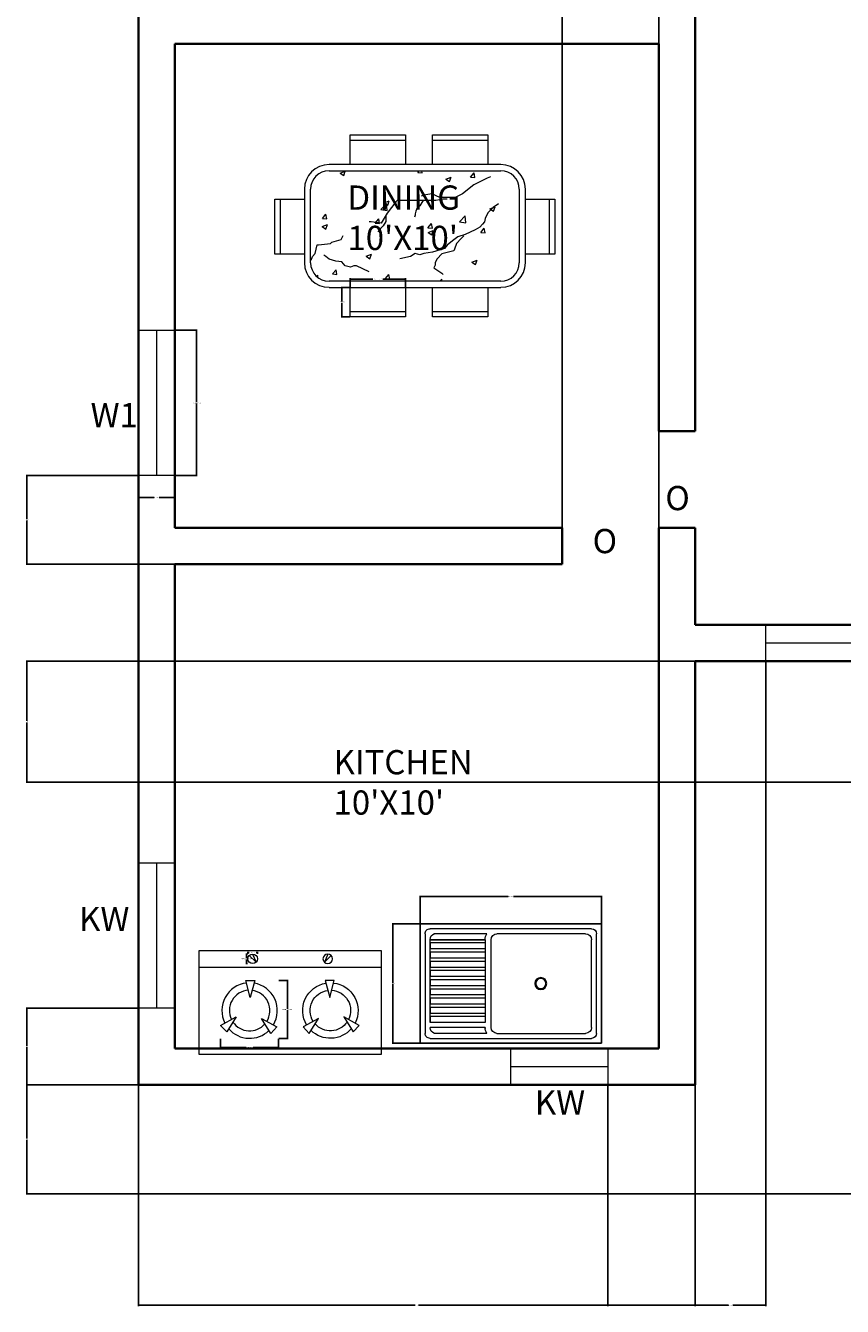
# Model space of a CAD drawing. Units: inches. Extents: x -4347 to -3836, y 955 to 1521.
# Tile 1 of 11: x -4347 to -4144, y 967 to 1284. Entities that reach past the tile are written whole.
import ezdxf

# ---------------------------------------------------------------- set-up
doc = ezdxf.new("R2010")
doc.units = ezdxf.units.IN
doc.header["$MEASUREMENT"] = 0
for name, color, linetype, lineweight in [('A-ANNO-DIMS', 2, 'Continuous', 18), ('A-ANNO-TEXT', 7, 'Continuous', 18), ('A-AREA-IDEN', 7, 'Continuous', 18), ('A-EQPM', 9, 'Continuous', 18), ('A-FLOR', 7, 'Continuous', 25), ('A-FLOR-FIXT', 9, 'Continuous', 18), ('A-FURN', 8, 'Continuous', 13), ('A-GLAZ', 4, 'Continuous', 18), ('A-WALL', 7, 'Continuous', 35)]:
    doc.layers.add(name, color=color, linetype=linetype, lineweight=lineweight)
doc.styles.get("Standard").update_dxf_attribs({"font": 'arial.ttf'})
doc.dimstyles.get("Standard").update_dxf_attribs({"dimtxt": 0.18, "dimasz": 0.18, "dimexe": 0.18, "dimexo": 0.0625, "dimgap": 0.09, "dimtad": 0, "dimtih": 1, "dimtoh": 1, "dimdec": 0, "dimzin": 0, "dimdsep": 46, "dimlunit": 3, "dimtxsty": 'Standard', "dimcen": 0.09, "dimadec": 0, "dimazin": 0, "dimtfac": 1, "dimtdec": 0, "dimtofl": 0, "dimtmove": 0, "dimatfit": 3, "dimfxl": 1, "dimtolj": 1, "dimtzin": 0, "dimarcsym": 0})

# ---------------------------------------------------------------- blocks, each defined once
blk = doc.blocks.new('М12 540х820')
for p, q in [((0, 540), (-820, 540)), ((-820, 540), (-820, 0)), ((0, 0), (0, 540)), ((-797.5, 495), (-797.5, 45)), ((-45, 517.5), (-775, 517.5)), ((-775, 468), (-775, 72)), ((-347.5, 495), (-748, 495)), ((-320.5, 468), (-320.5, 72)), ((-301.7, 495), (-64.8, 495)), ((-293.7, 468), (-293.7, 472.5)), ((-293.7, 468), (-45, 468)), ((-45, 469.5), (-45, 468)), ((-22.5, 45), (-22.5, 495)), ((-293.7, 446.6), (-45, 446.6)), ((-293.7, 419.6), (-293.7, 446.6)), ((-293.7, 419.6), (-45, 419.6)), ((-293.7, 405), (-45, 405)), ((-293.7, 378), (-293.7, 405)), ((-45, 419.6), (-45, 446.6)), ((-45, 378), (-45, 405)), ((-293.7, 378), (-45, 378)), ((-293.7, 336.4), (-293.7, 363.4)), ((-293.7, 363.4), (-45, 363.4)), ((-45, 336.4), (-45, 363.4)), ((-293.7, 336.4), (-45, 336.4)), ((-293.7, 294.7), (-293.7, 321.7)), ((-293.7, 321.7), (-45, 321.7)), ((-293.7, 294.7), (-45, 294.7)), ((-45, 294.7), (-45, 321.7)), ((-293.7, 253.1), (-293.7, 280.1)), ((-293.7, 280.1), (-45, 280.1)), ((-293.7, 253.1), (-45, 253.1)), ((-293.7, 211.5), (-293.7, 238.5)), ((-293.7, 238.5), (-45, 238.5)), ((-45, 253.1), (-45, 280.1)), ((-45, 211.5), (-45, 238.5)), ((-293.7, 211.5), (-45, 211.5)), ((-293.7, 169.9), (-293.7, 196.9)), ((-293.7, 196.9), (-45, 196.9)), ((-45, 169.9), (-45, 196.9)), ((-293.7, 169.9), (-45, 169.9)), ((-293.7, 128.2), (-293.7, 155.2)), ((-293.7, 155.2), (-45, 155.2)), ((-293.7, 128.2), (-45, 128.2)), ((-45, 128.2), (-45, 155.2)), ((-293.7, 113.6), (-45, 113.6)), ((-293.7, 86.6), (-293.7, 113.6)), ((-293.7, 86.6), (-45, 86.6)), ((-293.7, 72), (-45, 72)), ((-45, 86.6), (-45, 113.6)), ((-45, 70.5), (-45, 72)), ((-820, 0), (0, 0)), ((-775, 22.5), (-45, 22.5)), ((-748, 45), (-347.5, 45)), ((-301.7, 45), (-64.8, 45))]:
    blk.add_line(p, q)
at = {"ltscale": 0.06}
for p, q in [((-820, 0), (-820, 540)), ((-820, 540), (0, 540)), ((0, 540), (0, 536.9)), ((0, 536.9), (0, 0)), ((-293.7, 446.6), (-45, 446.6)), ((-293.7, 405), (-293.7, 446.6)), ((-293.7, 363.4), (-293.7, 405)), ((-45, 446.6), (-45, 419.6)), ((-45, 419.6), (-45, 378)), ((-293.7, 321.7), (-293.7, 363.4)), ((-45, 378), (-45, 336.4)), ((-293.7, 280.1), (-293.7, 321.7)), ((-45, 336.4), (-45, 294.7)), ((-45, 294.7), (-45, 253.1)), ((-293.7, 238.5), (-293.7, 280.1)), ((-293.7, 196.9), (-293.7, 238.5)), ((-45, 253.1), (-45, 211.5)), ((-293.7, 155.2), (-293.7, 196.9)), ((-45, 211.5), (-45, 169.9)), ((-293.7, 113.6), (-293.7, 155.2)), ((-45, 169.9), (-45, 128.2)), ((-45, 128.2), (-45, 86.6)), ((-293.7, 72), (-293.7, 113.6)), ((-45, 72), (-293.7, 72)), ((-45, 86.6), (-45, 72)), ((0, 0), (-820, 0))]:
    blk.add_line(p, q, dxfattribs=at)
at = {"extrusion": (0, 0, -1)}
for centre, major_axis, start_param, end_param in [((-775, 495), (-15.9, 15.9), -0.785398, 0.785398), ((-775, 495), (-15.9, 15.9), -0.785398, 0.785398), ((-748, 468), (-19.1, -19.1), 0.785398, 2.356194), ((-748, 468), (-19.1, -19.1), 0.785398, 2.356194), ((-347.5, 468), (-19.1, 19.1), 0.785398, 2.356194), ((-347.5, 468), (-19.1, 19.1), 0.785398, 2.356194), ((-343.2, 468), (-35, 35), 1.779263, 2.356194), ((-343.2, 468), (-35, 35), 1.779263, 2.356192), ((-343.2, 468), (-35, 35), 2.356192, 2.356194), ((-72.3, 468.8), (-19.3, 19.3), 1.0328, 2.38382), ((-72.3, 468.8), (-19.3, 19.3), 1.0328, 1.064673), ((-72.3, 468.8), (-19.3, 19.3), 1.064673, 2.328569), ((-45, 495), (-15.9, -15.9), 2.356194, 3.926991), ((-45, 495), (-15.9, -15.9), 2.356194, 3.926991), ((-72.3, 468.8), (-19.3, 19.3), 2.328569, 2.38382), ((-545.5, 270), (-19.1, -19.1), 3.926991, 10.210176), ((-545.5, 270), (-19.1, -19.1), 3.926991, 10.210176), ((-545.5, 270), (-15.9, -15.9), 3.926991, 10.210176), ((-545.5, 270), (-15.9, -15.9), 3.926991, 10.210176), ((-748, 72), (-19.1, 19.1), 3.926991, 5.497787), ((-748, 72), (-19.1, 19.1), 3.926991, 5.497787), ((-347.5, 72), (-19.1, -19.1), 3.926991, 5.497787), ((-347.5, 72), (-19.1, -19.1), 3.926991, 5.497787), ((-343.2, 72), (-35, -35), 3.926991, 4.503922), ((-343.2, 72), (-35, -35), 3.926991, 4.503922), ((-72.3, 71.2), (-19.3, -19.3), 3.899365, 5.250385), ((-72.3, 71.2), (-19.3, -19.3), 3.954617, 5.218512), ((-72.3, 71.2), (-19.3, -19.3), 3.899365, 3.954617), ((-775, 45), (-15.9, -15.9), 5.497787, 7.068583), ((-775, 45), (-15.9, -15.9), 5.497787, 7.068583), ((-72.3, 71.2), (-19.3, -19.3), 5.218512, 5.250385), ((-45, 45), (-15.9, 15.9), 2.356194, 3.926991), ((-45, 45), (-15.9, 15.9), 2.356194, 3.926991)]:
    blk.add_ellipse(centre, major_axis=major_axis, ratio=1, start_param=start_param, end_param=end_param, dxfattribs=at)
blk = doc.blocks.new('CHAIR-DINING')
for p, q in [((0, 0), (0, 7.33)), ((0, 7.33), (13.69, 7.33)), ((13.69, 7.33), (13.69, 0)), ((13.69, 5.99), (0, 5.99))]:
    blk.add_line(p, q)
blk = doc.blocks.new('GLAZ-24IN')
for p, q in [((0, 9), (24, 9)), ((0, 0), (0, 9)), ((24, 9), (24, 0)), ((0, 4.5), (24, 4.5)), ((24, 0), (0, 0))]:
    blk.add_line(p, q)
blk = doc.blocks.new('GLAZ-36IN')
for p, q in [((0, 0), (0, 36)), ((0, 36), (9, 36)), ((4.5, 36), (4.5, 0)), ((9, 36), (9, 0)), ((9, 0), (0, 0))]:
    blk.add_line(p, q)
blk = doc.blocks.new('GLAZ-60IN')
for p, q in [((0, 9), (60, 9)), ((0, 0), (0, 9)), ((60, 9), (60, 0)), ((0, 4.5), (60, 4.5)), ((60, 0), (0, 0))]:
    blk.add_line(p, q)
blk = doc.blocks.new('COOKTOP-BURNER')
for p, q in [((7.31, 10.12), (6.25, 14.36)), ((6.25, 14.36), (8.48, 14.36)), ((8.48, 14.36), (7.31, 10.12)), ((0, 3.2), (3.84, 5.33)), ((1.56, 1.61), (0, 3.2)), ((3.84, 5.33), (1.56, 1.61)), ((12.43, 1.2), (10.12, 4.94)), ((10.12, 4.94), (13.95, 2.83)), ((13.95, 2.83), (12.43, 1.2))]:
    blk.add_line(p, q)
for radius, start, end in [(6.87, 96.4005, 206.769), (6.87, 328.853, 80.7562), (5.03, 93.5753, 205.9207), (5.03, 327.9778, 83.02), (5.03, 214.5561, 318.8027), (6.87, 221.2225, 314.1627)]:
    blk.add_arc((7.18, 6.87), radius, start, end)
blk = doc.blocks.new('COOKTOP-CONTROL')
at = {"ltscale": 20}
for p, q in [((2.03, 0.35), (0.34, 2.02)), ((1.18, 2.37), (2.03, 0.35))]:
    blk.add_line(p, q, dxfattribs=at)
blk.add_circle((1.19, 1.19), 1.19, dxfattribs=at)
blk = doc.blocks.new('*D18')
at = {"layer": 'A-ANNO-DIMS', "color": 0, "lineweight": -2, "transparency": 16777216}
for p, q in [((-4266.08, 1219.49), (-4266.08, 1221.66)), ((-4265.9, 1221.48), (-4260.51, 1221.48)), ((-4252.57, 1221.48), (-4257.97, 1221.48)), ((-4252.39, 1219.49), (-4252.39, 1221.66))]:
    blk.add_line(p, q, dxfattribs=at)
at = {"layer": 'A-ANNO-DIMS', "color": 0, "transparency": 16777216}
for points in [[(-4265.9, 1221.51), (-4265.9, 1221.45), (-4266.08, 1221.48)], [(-4252.57, 1221.51), (-4252.57, 1221.45), (-4252.39, 1221.48)]]:
    blk.add_solid(points, dxfattribs=at)
at = {"layer": 'Defpoints', "color": 0, "transparency": 16777216}
for p in [(-4266.08, 1221.48), (-4266.08, 1219.42), (-4252.39, 1219.42)]:
    blk.add_point(p, dxfattribs=at)
at = {"layer": 'A-ANNO-DIMS', "color": 0, "transparency": 16777216, "insert": (-4259.24, 1221.48), "char_height": 0.18, "attachment_point": 5}
blk.add_mtext('\\A1;CHAIR 1\'-1 1/2" TYP.', dxfattribs=at)
blk = doc.blocks.new('*D19')
at = {"layer": 'A-ANNO-DIMS', "color": 0, "lineweight": -2, "transparency": 16777216}
for p, q in [((-4266.15, 1219.42), (-4268.32, 1219.42)), ((-4268.14, 1219.24), (-4268.14, 1215.94)), ((-4268.14, 1212.27), (-4268.14, 1215.57)), ((-4266.15, 1212.09), (-4268.32, 1212.09))]:
    blk.add_line(p, q, dxfattribs=at)
at = {"layer": 'A-ANNO-DIMS', "color": 0, "transparency": 16777216}
for points in [[(-4268.17, 1219.24), (-4268.11, 1219.24), (-4268.14, 1219.42)], [(-4268.17, 1212.27), (-4268.11, 1212.27), (-4268.14, 1212.09)]]:
    blk.add_solid(points, dxfattribs=at)
at = {"layer": 'Defpoints', "color": 0, "transparency": 16777216}
for p in [(-4266.08, 1219.42), (-4268.14, 1212.09), (-4266.08, 1212.09)]:
    blk.add_point(p, dxfattribs=at)
at = {"layer": 'A-ANNO-DIMS', "color": 0, "transparency": 16777216, "insert": (-4268.14, 1215.76), "char_height": 0.18, "attachment_point": 5}
blk.add_mtext('\\A1;0\'-7 1/2" TYP.', dxfattribs=at)
blk = doc.blocks.new('*D26')
at = {"layer": 'A-ANNO-DIMS', "color": 0, "lineweight": -2, "transparency": 16777216}
for p, q in [((-4309.52, 1208.78), (-4304, 1208.78)), ((-4304.18, 1208.6), (-4304.18, 1190.97)), ((-4304.18, 1172.96), (-4304.18, 1190.6)), ((-4309.52, 1172.78), (-4304, 1172.78))]:
    blk.add_line(p, q, dxfattribs=at)
at = {"layer": 'A-ANNO-DIMS', "color": 0, "transparency": 16777216}
for points in [[(-4304.21, 1208.6), (-4304.15, 1208.6), (-4304.18, 1208.78)], [(-4304.21, 1172.96), (-4304.15, 1172.96), (-4304.18, 1172.78)]]:
    blk.add_solid(points, dxfattribs=at)
at = {"layer": 'Defpoints', "color": 0, "transparency": 16777216}
for p in [(-4309.58, 1208.78), (-4304.18, 1208.78), (-4309.58, 1172.78)]:
    blk.add_point(p, dxfattribs=at)
at = {"layer": 'A-ANNO-DIMS', "color": 0, "transparency": 16777216, "insert": (-4304.18, 1190.78), "char_height": 0.18, "attachment_point": 5}
blk.add_mtext('\\A1;GLAZING 3\'-0" TYP.', dxfattribs=at)
blk = doc.blocks.new('*D27')
at = {"layer": 'A-ANNO-DIMS', "color": 0, "lineweight": -2, "transparency": 16777216}
for p, q in [((-4318.58, 1172.72), (-4318.58, 1167.2)), ((-4309.58, 1172.72), (-4309.58, 1167.2)), ((-4318.4, 1167.38), (-4314.72, 1167.38)), ((-4309.76, 1167.38), (-4313.44, 1167.38))]:
    blk.add_line(p, q, dxfattribs=at)
at = {"layer": 'A-ANNO-DIMS', "color": 0, "transparency": 16777216}
for points in [[(-4318.4, 1167.41), (-4318.4, 1167.35), (-4318.58, 1167.38)], [(-4309.76, 1167.41), (-4309.76, 1167.35), (-4309.58, 1167.38)]]:
    blk.add_solid(points, dxfattribs=at)
at = {"layer": 'Defpoints', "color": 0, "transparency": 16777216}
for p in [(-4318.58, 1172.78), (-4309.58, 1172.78), (-4309.58, 1167.38)]:
    blk.add_point(p, dxfattribs=at)
at = {"layer": 'A-ANNO-DIMS', "color": 0, "transparency": 16777216, "insert": (-4314.08, 1167.38), "char_height": 0.18, "attachment_point": 5}
blk.add_mtext('\\A1;0\'-9" TYP.', dxfattribs=at)
blk = doc.blocks.new('*D30')
at = {"layer": 'A-ANNO-DIMS', "color": 0, "lineweight": -2, "transparency": 16777216}
for p, q in [((-4283.77, 1047.67), (-4281.48, 1047.67)), ((-4281.66, 1047.49), (-4281.66, 1040.63)), ((-4281.66, 1033.41), (-4281.66, 1040.27)), ((-4283.77, 1033.23), (-4281.48, 1033.23))]:
    blk.add_line(p, q, dxfattribs=at)
at = {"layer": 'A-ANNO-DIMS', "color": 0, "transparency": 16777216}
for points in [[(-4281.69, 1047.49), (-4281.63, 1047.49), (-4281.66, 1047.67)], [(-4281.69, 1033.41), (-4281.63, 1033.41), (-4281.66, 1033.23)]]:
    blk.add_solid(points, dxfattribs=at)
at = {"layer": 'Defpoints', "color": 0, "transparency": 16777216}
for p in [(-4283.83, 1047.67), (-4281.66, 1047.67), (-4283.83, 1033.23)]:
    blk.add_point(p, dxfattribs=at)
at = {"layer": 'A-ANNO-DIMS', "color": 0, "transparency": 16777216, "insert": (-4281.66, 1040.45), "char_height": 0.18, "attachment_point": 5}
blk.add_mtext('\\A1;BURNER 1\'-2 1/2" TYP.', dxfattribs=at)
blk = doc.blocks.new('*D31')
at = {"layer": 'A-ANNO-DIMS', "color": 0, "lineweight": -2, "transparency": 16777216}
for p, q in [((-4298.21, 1033.17), (-4298.21, 1030.89)), ((-4283.83, 1033.17), (-4283.83, 1030.89)), ((-4298.03, 1031.07), (-4291.86, 1031.07)), ((-4284.01, 1031.07), (-4290.18, 1031.07))]:
    blk.add_line(p, q, dxfattribs=at)
at = {"layer": 'A-ANNO-DIMS', "color": 0, "transparency": 16777216}
for points in [[(-4298.03, 1031.1), (-4298.03, 1031.04), (-4298.21, 1031.07)], [(-4284.01, 1031.1), (-4284.01, 1031.04), (-4283.83, 1031.07)]]:
    blk.add_solid(points, dxfattribs=at)
at = {"layer": 'Defpoints', "color": 0, "transparency": 16777216}
for p in [(-4298.21, 1033.23), (-4283.83, 1033.23), (-4283.83, 1031.07)]:
    blk.add_point(p, dxfattribs=at)
at = {"layer": 'A-ANNO-DIMS', "color": 0, "transparency": 16777216, "insert": (-4291.02, 1031.07), "char_height": 0.18, "attachment_point": 5}
blk.add_mtext('\\A1;1\'-2 1/2" TYP.', dxfattribs=at)
blk = doc.blocks.new('*D32')
at = {"layer": 'A-ANNO-DIMS', "color": 0, "lineweight": -2, "transparency": 16777216}
for p, q in [((-4291.53, 1054.2), (-4292.01, 1054.2)), ((-4291.83, 1054.02), (-4291.83, 1053.19)), ((-4291.53, 1051.82), (-4292.01, 1051.82)), ((-4291.83, 1052), (-4291.83, 1052.83))]:
    blk.add_line(p, q, dxfattribs=at)
at = {"layer": 'A-ANNO-DIMS', "color": 0, "transparency": 16777216}
for points in [[(-4291.86, 1054.02), (-4291.8, 1054.02), (-4291.83, 1054.2)], [(-4291.86, 1052), (-4291.8, 1052), (-4291.83, 1051.82)]]:
    blk.add_solid(points, dxfattribs=at)
at = {"layer": 'Defpoints', "color": 0, "transparency": 16777216}
for p in [(-4291.83, 1054.2), (-4291.47, 1054.2), (-4291.47, 1051.82)]:
    blk.add_point(p, dxfattribs=at)
at = {"layer": 'A-ANNO-DIMS', "color": 0, "transparency": 16777216, "insert": (-4291.83, 1053.01), "char_height": 0.18, "attachment_point": 5}
blk.add_mtext('\\A1;CONTROL 0\'-2 1/2" TYP.', dxfattribs=at)
blk = doc.blocks.new('*D33')
at = {"layer": 'A-ANNO-DIMS', "color": 0, "lineweight": -2, "transparency": 16777216}
for p, q in [((-4291.47, 1054.26), (-4291.47, 1054.73)), ((-4291.29, 1054.55), (-4291.13, 1054.55)), ((-4289.28, 1054.55), (-4289.44, 1054.55)), ((-4289.1, 1054.26), (-4289.1, 1054.73))]:
    blk.add_line(p, q, dxfattribs=at)
at = {"layer": 'A-ANNO-DIMS', "color": 0, "transparency": 16777216}
for points in [[(-4291.29, 1054.58), (-4291.29, 1054.52), (-4291.47, 1054.55)], [(-4289.28, 1054.58), (-4289.28, 1054.52), (-4289.1, 1054.55)]]:
    blk.add_solid(points, dxfattribs=at)
at = {"layer": 'Defpoints', "color": 0, "transparency": 16777216}
for p in [(-4291.47, 1054.2), (-4289.1, 1054.55), (-4289.1, 1054.2)]:
    blk.add_point(p, dxfattribs=at)
at = {"layer": 'A-ANNO-DIMS', "color": 0, "transparency": 16777216, "insert": (-4290.28, 1054.55), "char_height": 0.18, "attachment_point": 5}
blk.add_mtext('\\A1;0\'-2 1/2" TYP.', dxfattribs=at)
blk = doc.blocks.new('*D34')
at = {"layer": 'A-ANNO-DIMS', "color": 0, "lineweight": -2, "transparency": 16777216}
for p, q in [((-4248.77, 1061.76), (-4248.77, 1068.63)), ((-4248.59, 1068.45), (-4226.92, 1068.45)), ((-4203.95, 1068.45), (-4225.61, 1068.45)), ((-4203.77, 1061.76), (-4203.77, 1068.63))]:
    blk.add_line(p, q, dxfattribs=at)
at = {"layer": 'A-ANNO-DIMS', "color": 0, "transparency": 16777216}
for points in [[(-4248.59, 1068.48), (-4248.59, 1068.42), (-4248.77, 1068.45)], [(-4203.95, 1068.48), (-4203.95, 1068.42), (-4203.77, 1068.45)]]:
    blk.add_solid(points, dxfattribs=at)
at = {"layer": 'Defpoints', "color": 0, "transparency": 16777216}
for p in [(-4248.77, 1068.45), (-4248.77, 1061.7), (-4203.77, 1061.7)]:
    blk.add_point(p, dxfattribs=at)
at = {"layer": 'A-ANNO-DIMS', "color": 0, "transparency": 16777216, "insert": (-4226.27, 1068.45), "char_height": 0.18, "attachment_point": 5}
blk.add_mtext('\\A1;SINK 3\'-9"', dxfattribs=at)
blk = doc.blocks.new('*D35')
at = {"layer": 'A-ANNO-DIMS', "color": 0, "lineweight": -2, "transparency": 16777216}
for p, q in [((-4248.83, 1061.7), (-4255.7, 1061.7)), ((-4255.52, 1061.52), (-4255.52, 1047.07)), ((-4255.52, 1032.25), (-4255.52, 1046.7)), ((-4248.83, 1032.07), (-4255.7, 1032.07))]:
    blk.add_line(p, q, dxfattribs=at)
at = {"layer": 'A-ANNO-DIMS', "color": 0, "transparency": 16777216}
for points in [[(-4255.55, 1061.52), (-4255.49, 1061.52), (-4255.52, 1061.7)], [(-4255.55, 1032.25), (-4255.49, 1032.25), (-4255.52, 1032.07)]]:
    blk.add_solid(points, dxfattribs=at)
at = {"layer": 'Defpoints', "color": 0, "transparency": 16777216}
for p in [(-4248.77, 1061.7), (-4255.52, 1032.07), (-4248.77, 1032.07)]:
    blk.add_point(p, dxfattribs=at)
at = {"layer": 'A-ANNO-DIMS', "color": 0, "transparency": 16777216, "insert": (-4255.52, 1046.88), "char_height": 0.18, "attachment_point": 5}
blk.add_mtext('\\A1;2\'-5 1/2"', dxfattribs=at)
blk = doc.blocks.new('*D39')
at = {"layer": 'A-ANNO-DIMS', "color": 0, "lineweight": -2, "transparency": 16777216}
for p, q in [((-4318.58, 1021.73), (-4318.58, 966.96)), ((-4180.58, 1021.73), (-4180.58, 966.96)), ((-4318.4, 967.14), (-4249.97, 967.14)), ((-4180.76, 967.14), (-4249.19, 967.14))]:
    blk.add_line(p, q, dxfattribs=at)
at = {"layer": 'A-ANNO-DIMS', "color": 0, "transparency": 16777216}
for points in [[(-4318.4, 967.17), (-4318.4, 967.11), (-4318.58, 967.14)], [(-4180.76, 967.17), (-4180.76, 967.11), (-4180.58, 967.14)]]:
    blk.add_solid(points, dxfattribs=at)
at = {"layer": 'Defpoints', "color": 0, "transparency": 16777216}
for p in [(-4318.58, 1021.79), (-4180.58, 1021.79), (-4180.58, 967.14)]:
    blk.add_point(p, dxfattribs=at)
at = {"layer": 'A-ANNO-DIMS', "color": 0, "transparency": 16777216, "insert": (-4249.58, 967.14), "char_height": 0.18, "attachment_point": 5}
blk.add_mtext('\\A1;11\'-6"', dxfattribs=at)
blk = doc.blocks.new('*D40')
at = {"layer": 'A-ANNO-DIMS', "color": 0, "lineweight": -2, "transparency": 16777216}
for p, q in [((-4318.64, 1021.79), (-4346.41, 1021.79)), ((-4346.23, 1021.61), (-4346.23, 1008.47)), ((-4346.23, 994.97), (-4346.23, 1008.11)), ((-4180.64, 994.79), (-4346.41, 994.79))]:
    blk.add_line(p, q, dxfattribs=at)
at = {"layer": 'A-ANNO-DIMS', "color": 0, "transparency": 16777216}
for points in [[(-4346.26, 1021.61), (-4346.2, 1021.61), (-4346.23, 1021.79)], [(-4346.26, 994.97), (-4346.2, 994.97), (-4346.23, 994.79)]]:
    blk.add_solid(points, dxfattribs=at)
at = {"layer": 'Defpoints', "color": 0, "transparency": 16777216}
for p in [(-4346.23, 1021.79), (-4318.58, 1021.79), (-4180.58, 994.79)]:
    blk.add_point(p, dxfattribs=at)
at = {"layer": 'A-ANNO-DIMS', "color": 0, "transparency": 16777216, "insert": (-4346.23, 1008.29), "char_height": 0.18, "attachment_point": 5}
blk.add_mtext('\\A1;2\'-3"', dxfattribs=at)
blk = doc.blocks.new('*D41')
at = {"layer": 'A-ANNO-DIMS', "color": 0, "lineweight": -2, "transparency": 16777216}
for p, q in [((-4318.64, 1040.78), (-4346.41, 1040.78)), ((-4346.23, 1040.6), (-4346.23, 1031.46)), ((-4346.23, 1021.97), (-4346.23, 1031.1)), ((-4318.64, 1021.79), (-4346.41, 1021.79))]:
    blk.add_line(p, q, dxfattribs=at)
at = {"layer": 'A-ANNO-DIMS', "color": 0, "transparency": 16777216}
for points in [[(-4346.26, 1040.6), (-4346.2, 1040.6), (-4346.23, 1040.78)], [(-4346.26, 1021.97), (-4346.2, 1021.97), (-4346.23, 1021.79)]]:
    blk.add_solid(points, dxfattribs=at)
at = {"layer": 'Defpoints', "color": 0, "transparency": 16777216}
for p in [(-4346.23, 1040.78), (-4318.58, 1040.78), (-4318.58, 1021.79)]:
    blk.add_point(p, dxfattribs=at)
at = {"layer": 'A-ANNO-DIMS', "color": 0, "transparency": 16777216, "insert": (-4346.23, 1031.28), "char_height": 0.18, "attachment_point": 5}
blk.add_mtext('\\A1;1\'-7"', dxfattribs=at)
blk = doc.blocks.new('*D42')
at = {"layer": 'A-ANNO-DIMS', "color": 0, "lineweight": -2, "transparency": 16777216}
for p, q in [((-4318.64, 1172.78), (-4346.41, 1172.78)), ((-4346.23, 1172.6), (-4346.23, 1161.97)), ((-4346.23, 1150.97), (-4346.23, 1161.6)), ((-4309.64, 1150.79), (-4346.41, 1150.79))]:
    blk.add_line(p, q, dxfattribs=at)
at = {"layer": 'A-ANNO-DIMS', "color": 0, "transparency": 16777216}
for points in [[(-4346.26, 1172.6), (-4346.2, 1172.6), (-4346.23, 1172.78)], [(-4346.26, 1150.97), (-4346.2, 1150.97), (-4346.23, 1150.79)]]:
    blk.add_solid(points, dxfattribs=at)
at = {"layer": 'Defpoints', "color": 0, "transparency": 16777216}
for p in [(-4346.23, 1172.78), (-4318.58, 1172.78), (-4309.58, 1150.79)]:
    blk.add_point(p, dxfattribs=at)
at = {"layer": 'A-ANNO-DIMS', "color": 0, "transparency": 16777216, "insert": (-4346.23, 1161.79), "char_height": 0.18, "attachment_point": 5}
blk.add_mtext('\\A1;1\'-10"', dxfattribs=at)
blk = doc.blocks.new('*D46')
at = {"layer": 'A-ANNO-DIMS', "color": 0, "lineweight": -2, "transparency": 16777216}
for p, q in [((-4202.26, 1021.73), (-4202.26, 966.96)), ((-4180.58, 1021.73), (-4180.58, 966.96)), ((-4202.08, 967.14), (-4191.95, 967.14)), ((-4180.76, 967.14), (-4190.89, 967.14))]:
    blk.add_line(p, q, dxfattribs=at)
at = {"layer": 'A-ANNO-DIMS', "color": 0, "transparency": 16777216}
for points in [[(-4202.08, 967.17), (-4202.08, 967.11), (-4202.26, 967.14)], [(-4180.76, 967.17), (-4180.76, 967.11), (-4180.58, 967.14)]]:
    blk.add_solid(points, dxfattribs=at)
at = {"layer": 'Defpoints', "color": 0, "transparency": 16777216}
for p in [(-4202.26, 1021.79), (-4180.58, 1021.79), (-4180.58, 967.14)]:
    blk.add_point(p, dxfattribs=at)
at = {"layer": 'A-ANNO-DIMS', "color": 0, "transparency": 16777216, "insert": (-4191.42, 967.14), "char_height": 0.18, "attachment_point": 5}
blk.add_mtext('\\A1;1\'-9 1/2"', dxfattribs=at)
blk = doc.blocks.new('*D54')
at = {"layer": 'A-ANNO-DIMS', "color": 0, "lineweight": -2, "transparency": 16777216}
for p, q in [((-3997.76, 1126.79), (-4346.41, 1126.79)), ((-4346.23, 1126.61), (-4346.23, 1111.97)), ((-4346.23, 1096.97), (-4346.23, 1111.61)), ((-3997.76, 1096.79), (-4346.41, 1096.79))]:
    blk.add_line(p, q, dxfattribs=at)
at = {"layer": 'A-ANNO-DIMS', "color": 0, "transparency": 16777216}
for points in [[(-4346.26, 1126.61), (-4346.2, 1126.61), (-4346.23, 1126.79)], [(-4346.26, 1096.97), (-4346.2, 1096.97), (-4346.23, 1096.79)]]:
    blk.add_solid(points, dxfattribs=at)
at = {"layer": 'Defpoints', "color": 0, "transparency": 16777216}
for p in [(-4346.23, 1126.79), (-3997.69, 1126.79), (-3997.69, 1096.79)]:
    blk.add_point(p, dxfattribs=at)
at = {"layer": 'A-ANNO-DIMS', "color": 0, "transparency": 16777216, "insert": (-4346.23, 1111.79), "char_height": 0.18, "attachment_point": 5}
blk.add_mtext('\\A1;2\'-6"', dxfattribs=at)
blk = doc.blocks.new('*D56')
at = {"layer": 'A-ANNO-DIMS', "color": 0, "lineweight": -2, "transparency": 16777216}
for p, q in [((-4180.58, 1126.73), (-4180.58, 966.96)), ((-4163.03, 1126.73), (-4163.03, 966.96)), ((-4180.4, 967.14), (-4172.34, 967.14)), ((-4163.21, 967.14), (-4171.27, 967.14))]:
    blk.add_line(p, q, dxfattribs=at)
at = {"layer": 'A-ANNO-DIMS', "color": 0, "transparency": 16777216}
for points in [[(-4180.4, 967.17), (-4180.4, 967.11), (-4180.58, 967.14)], [(-4163.21, 967.17), (-4163.21, 967.11), (-4163.03, 967.14)]]:
    blk.add_solid(points, dxfattribs=at)
at = {"layer": 'Defpoints', "color": 0, "transparency": 16777216}
for p in [(-4180.58, 1126.79), (-4163.03, 1126.79), (-4163.03, 967.14)]:
    blk.add_point(p, dxfattribs=at)
at = {"layer": 'A-ANNO-DIMS', "color": 0, "transparency": 16777216, "insert": (-4171.81, 967.14), "char_height": 0.18, "attachment_point": 5}
blk.add_mtext('\\A1;1\'-5 1/2"', dxfattribs=at)
blk = doc.blocks.new('*D58')
at = {"layer": 'A-ANNO-DIMS', "color": 0, "lineweight": -2, "transparency": 16777216}
for p, q in [((-4213.58, 1159.85), (-4213.58, 1517.62)), ((-4213.4, 1517.44), (-4201.91, 1517.44)), ((-4189.76, 1517.44), (-4201.25, 1517.44)), ((-4189.58, 1159.85), (-4189.58, 1517.62))]:
    blk.add_line(p, q, dxfattribs=at)
at = {"layer": 'A-ANNO-DIMS', "color": 0, "transparency": 16777216}
for points in [[(-4213.4, 1517.47), (-4213.4, 1517.41), (-4213.58, 1517.44)], [(-4189.76, 1517.47), (-4189.76, 1517.41), (-4189.58, 1517.44)]]:
    blk.add_solid(points, dxfattribs=at)
at = {"layer": 'Defpoints', "color": 0, "transparency": 16777216}
for p in [(-4189.58, 1517.44), (-4213.58, 1159.79), (-4189.58, 1159.79)]:
    blk.add_point(p, dxfattribs=at)
at = {"layer": 'A-ANNO-DIMS', "color": 0, "transparency": 16777216, "insert": (-4201.58, 1517.44), "char_height": 0.18, "attachment_point": 5}
blk.add_mtext('\\A1;2\'-0"', dxfattribs=at)

msp = doc.modelspace()

# ---------------------------------------------------------------- linework, layer by layer
at = {"layer": 'A-EQPM'}
msp.add_line((-4303.51, 1050.91), (-4258.42, 1050.91), dxfattribs=at)
msp.add_lwpolyline([(-4258.42, 1029.33), (-4303.51, 1029.33), (-4303.51, 1055.1), (-4258.42, 1055.1)], close=True, dxfattribs=at)
at = {"layer": 'A-FLOR'}
for p, q in [((-4180.58, 1021.79), (-4180.58, 994.79)), ((-4180.58, 994.79), (-3931.58, 994.79))]:
    msp.add_line(p, q, dxfattribs=at)
at = {"layer": 'A-FURN'}
for p, q in [((-4228.75, 1249.85), (-4271.35, 1249.85)), ((-4271.35, 1248.33), (-4228.75, 1248.33)), ((-4268.58, 1247.72), (-4267.31, 1248.21)), ((-4268.58, 1247.72), (-4267.68, 1247.11)), ((-4267.68, 1247.11), (-4267.31, 1248.21)), ((-4249.34, 1247.91), (-4248.99, 1248.33)), ((-4249.34, 1247.91), (-4248.25, 1247.81)), ((-4248.25, 1247.81), (-4248.35, 1248.33)), ((-4236.25, 1246.76), (-4235.37, 1247.81)), ((-4235.16, 1246.67), (-4235.37, 1247.81)), ((-4242.35, 1246.26), (-4241.07, 1246.75)), ((-4242.35, 1246.26), (-4241.44, 1245.64)), ((-4241.44, 1245.64), (-4241.07, 1246.75)), ((-4235.44, 1244.87), (-4238.25, 1242.56)), ((-4236.25, 1246.76), (-4235.16, 1246.67)), ((-4232.13, 1246.52), (-4235.44, 1244.87)), ((-4231.3, 1246.85), (-4232.13, 1246.52)), ((-4277.43, 1243.76), (-4277.43, 1225.51)), ((-4275.91, 1225.51), (-4275.91, 1243.76)), ((-4247.84, 1242.23), (-4248.5, 1242.06)), ((-4245.86, 1242.56), (-4247.84, 1242.23)), ((-4243.87, 1241.73), (-4245.86, 1242.56)), ((-4243.05, 1241.24), (-4244.86, 1240.91)), ((-4240.07, 1241.73), (-4243.87, 1241.73)), ((-4242.05, 1241.24), (-4243.05, 1241.24)), ((-4238.25, 1242.56), (-4240.07, 1241.73)), ((-4224.19, 1243.76), (-4224.19, 1225.51)), ((-4222.67, 1225.51), (-4222.67, 1243.76)), ((-4258.51, 1238.71), (-4257.09, 1240.19)), ((-4258.51, 1238.71), (-4256.89, 1238.46)), ((-4257.69, 1240.37), (-4256.41, 1240.86)), ((-4257.69, 1240.37), (-4256.78, 1239.76)), ((-4256.89, 1238.46), (-4257.09, 1240.19)), ((-4254.79, 1240.58), (-4256.94, 1237.77)), ((-4256.78, 1239.76), (-4256.41, 1240.86)), ((-4254.46, 1240.91), (-4254.79, 1240.58)), ((-4244.86, 1240.91), (-4254.46, 1240.91)), ((-4249.83, 1238.27), (-4249.99, 1237.61)), ((-4249.49, 1239.09), (-4249.83, 1238.27)), ((-4248.83, 1239.59), (-4249.49, 1239.09)), ((-4248.34, 1240.42), (-4248.83, 1239.59)), ((-4248.01, 1240.91), (-4248.34, 1240.42)), ((-4231.96, 1237.93), (-4232.62, 1236.45)), ((-4230.64, 1239.25), (-4231.96, 1237.93)), ((-4231.45, 1238.91), (-4230.18, 1239.4)), ((-4231.45, 1238.91), (-4230.55, 1238.29)), ((-4229.32, 1240.08), (-4230.64, 1239.25)), ((-4230.55, 1238.29), (-4230.18, 1239.4)), ((-4273.03, 1234.48), (-4271.75, 1234.97)), ((-4273, 1236.47), (-4272.12, 1237.52)), ((-4273, 1236.47), (-4271.91, 1236.37)), ((-4271.91, 1236.37), (-4272.12, 1237.52)), ((-4272.12, 1233.87), (-4271.75, 1234.97)), ((-4260.91, 1235.62), (-4261.41, 1235.62)), ((-4258.43, 1235.29), (-4260.91, 1235.62)), ((-4259.9, 1235.32), (-4259.02, 1236.37)), ((-4259.9, 1235.32), (-4258.81, 1235.23)), ((-4258.81, 1235.23), (-4259.02, 1236.37)), ((-4256.94, 1237.77), (-4258.43, 1235.29)), ((-4257.27, 1235.78), (-4257.93, 1234.63)), ((-4257.27, 1237.27), (-4257.27, 1235.78)), ((-4249.99, 1237.28), (-4250.16, 1236.78)), ((-4249.99, 1237.61), (-4249.99, 1237.28)), ((-4246.81, 1234.18), (-4245.93, 1235.23)), ((-4245.72, 1234.08), (-4245.93, 1235.22)), ((-4239.03, 1235.69), (-4237.6, 1237.17)), ((-4239.03, 1235.69), (-4237.4, 1235.44)), ((-4237.4, 1235.44), (-4237.6, 1237.17)), ((-4233.29, 1235.12), (-4233.95, 1234.3)), ((-4232.79, 1235.62), (-4233.29, 1235.12)), ((-4232.62, 1236.45), (-4232.79, 1235.62)), ((-4273.03, 1234.48), (-4272.12, 1233.87)), ((-4268.35, 1231.32), (-4267.86, 1232.31)), ((-4258.59, 1233.97), (-4259.26, 1233.14)), ((-4257.93, 1234.63), (-4258.59, 1233.97)), ((-4246.81, 1234.18), (-4245.72, 1234.08)), ((-4246.79, 1233.02), (-4245.51, 1233.51)), ((-4246.79, 1233.02), (-4245.88, 1232.41)), ((-4245.88, 1232.41), (-4245.51, 1233.51)), ((-4239.41, 1231.98), (-4240.73, 1230.99)), ((-4237.59, 1232.48), (-4239.41, 1231.98)), ((-4237.92, 1232.15), (-4238.58, 1231.49)), ((-4235.11, 1233.64), (-4237.59, 1232.48)), ((-4233.95, 1234.3), (-4235.11, 1233.64)), ((-4233.72, 1233.03), (-4232.84, 1234.08)), ((-4233.72, 1233.03), (-4232.63, 1232.94)), ((-4232.62, 1232.93), (-4232.84, 1234.08)), ((-4274.8, 1227.85), (-4274.31, 1230)), ((-4274.31, 1230), (-4273.98, 1230)), ((-4273.98, 1230), (-4271, 1230.33)), ((-4271, 1230.33), (-4270.67, 1230.66)), ((-4270.67, 1230.66), (-4268.35, 1231.32)), ((-4242.71, 1229.01), (-4245.69, 1228.18)), ((-4240.4, 1228.51), (-4243.38, 1227.69)), ((-4242.05, 1229.84), (-4242.71, 1229.01)), ((-4240.73, 1230.99), (-4242.05, 1229.84)), ((-4240.23, 1228.85), (-4240.4, 1228.51)), ((-4239.74, 1230.33), (-4240.23, 1228.85)), ((-4238.58, 1231.49), (-4239.74, 1230.33)), ((-4275.8, 1226.2), (-4275.47, 1227.03)), ((-4275.47, 1227.03), (-4274.8, 1227.85)), ((-4272.16, 1227.03), (-4272.65, 1227.36)), ((-4271.33, 1226.37), (-4272.16, 1227.03)), ((-4269.67, 1225.88), (-4271.33, 1226.37)), ((-4268.19, 1225.71), (-4269.67, 1225.88)), ((-4267.36, 1224.72), (-4268.19, 1225.71)), ((-4262.13, 1227.13), (-4260.85, 1227.62)), ((-4262.13, 1227.13), (-4261.22, 1226.52)), ((-4261.22, 1226.52), (-4260.85, 1227.62)), ((-4251.15, 1227.03), (-4253.8, 1226.53)), ((-4249.99, 1227.85), (-4251.15, 1227.03)), ((-4248.83, 1227.52), (-4249.99, 1227.85)), ((-4247.84, 1227.85), (-4248.83, 1227.52)), ((-4245.69, 1228.18), (-4247.84, 1227.85)), ((-4244.53, 1226.53), (-4245.03, 1225.54)), ((-4245.03, 1225.54), (-4245.03, 1224.88)), ((-4243.38, 1227.69), (-4244.53, 1226.53)), ((-4235.9, 1225.67), (-4234.62, 1226.16)), ((-4235.9, 1225.67), (-4234.99, 1225.06)), ((-4234.99, 1225.06), (-4234.62, 1226.16)), ((-4274.42, 1222.13), (-4274.15, 1222.41)), ((-4274.08, 1221.86), (-4274.15, 1222.41)), ((-4270.46, 1222.74), (-4269.58, 1223.79)), ((-4270.46, 1222.74), (-4269.37, 1222.64)), ((-4269.37, 1222.64), (-4269.58, 1223.78)), ((-4266.04, 1224.39), (-4267.36, 1224.72)), ((-4265.21, 1224.72), (-4266.04, 1224.39)), ((-4264.55, 1224.72), (-4265.21, 1224.72)), ((-4261.4, 1223.23), (-4264.55, 1224.72)), ((-4257.37, 1221.59), (-4256.49, 1222.64)), ((-4256.28, 1221.49), (-4256.49, 1222.64)), ((-4245.03, 1224.88), (-4245.36, 1224.22)), ((-4245.36, 1224.22), (-4243.38, 1222.9)), ((-4243.38, 1222.9), (-4243.05, 1222.57)), ((-4228.75, 1220.94), (-4271.35, 1220.94)), ((-4271.35, 1219.42), (-4228.75, 1219.42)), ((-4257.37, 1221.59), (-4256.28, 1221.5)), ((-4243.86, 1220.94), (-4243.4, 1221.49)), ((-4243.3, 1220.94), (-4243.4, 1221.49))]:
    msp.add_line(p, q, dxfattribs=at)
for centre, radius, start, end in [((-4271.35, 1243.76), 6.08, 90, 180), ((-4271.35, 1243.76), 4.56, 90, 180), ((-4228.75, 1243.76), 6.08, 0, 90), ((-4228.75, 1243.76), 4.56, 0, 90), ((-4271.35, 1225.51), 6.08, 180, 270), ((-4271.35, 1225.51), 4.56, 180, 270), ((-4228.75, 1225.51), 4.56, 270, 0), ((-4228.75, 1225.51), 6.08, 270, 0)]:
    msp.add_arc(centre, radius, start, end, dxfattribs=at)
at = {"layer": 'A-WALL'}
for p, q in [((-4318.58, 1489.79), (-4318.58, 1021.79)), ((-4180.58, 1348.79), (-4180.58, 1183.79)), ((-4309.58, 1279.79), (-4189.58, 1279.79)), ((-4309.58, 1279.79), (-4309.58, 1159.79)), ((-4189.58, 1279.79), (-4189.58, 1183.79)), ((-4180.58, 1183.79), (-4189.58, 1183.79)), ((-4309.58, 1159.79), (-4213.58, 1159.79)), ((-4213.58, 1159.79), (-4213.58, 1150.79)), ((-4189.58, 1159.79), (-4180.58, 1159.79)), ((-4189.58, 1159.79), (-4189.58, 1030.79)), ((-4180.58, 1159.79), (-4180.58, 1135.79)), ((-4309.58, 1150.79), (-4213.58, 1150.79)), ((-4309.58, 1150.79), (-4309.58, 1030.79)), ((-4180.58, 1135.79), (-3976.58, 1135.79)), ((-4180.58, 1126.79), (-3976.58, 1126.79)), ((-4180.58, 1126.79), (-4180.58, 1021.79)), ((-4309.58, 1030.79), (-4189.58, 1030.79)), ((-4318.58, 1021.79), (-4180.58, 1021.79))]:
    msp.add_line(p, q, dxfattribs=at)

# ---------------------------------------------------------------- block references
at = {"layer": 'A-EQPM'}
for name, p in [('COOKTOP-CONTROL', (-4291.47, 1051.82)), ('COOKTOP-BURNER', (-4298.21, 1033.31))]:
    msp.add_blockref(name, p, dxfattribs=at)
at = {"layer": 'A-EQPM', "extrusion": (0, 0, -1), "zscale": -1}
for name, p in [('COOKTOP-CONTROL', (4270.46, 1051.82)), ('COOKTOP-BURNER', (4263.83, 1033.31))]:
    msp.add_blockref(name, p, dxfattribs=at)
at = {"layer": 'A-FLOR-FIXT', "xscale": 0.0548780487802039, "yscale": 0.0548780487802039, "zscale": 0.0548780487802039, "rotation": 180}
msp.add_blockref('М12 540х820', (-4248.77, 1061.7), dxfattribs=at)
at = {"layer": 'A-FURN'}
for p in [(-4266.09, 1249.85), (-4245.7, 1249.85)]:
    msp.add_blockref('CHAIR-DINING', p, dxfattribs=at)
for p, rotation in [((-4277.43, 1227.61), 89.9999999967525), ((-4222.67, 1241.3), 269.9999999873025), ((-4252.39, 1219.42), 180), ((-4232.01, 1219.42), 180)]:
    msp.add_blockref('CHAIR-DINING', p, dxfattribs=dict(at, rotation=rotation))
at = {"layer": 'A-GLAZ'}
for name, p in [('GLAZ-36IN', (-4318.58, 1172.78)), ('GLAZ-60IN', (-4163.03, 1126.79)), ('GLAZ-36IN', (-4318.58, 1040.78)), ('GLAZ-24IN', (-4226.26, 1021.79))]:
    msp.add_blockref(name, p, dxfattribs=at)

# ---------------------------------------------------------------- texts
at = {"layer": 'A-ANNO-TEXT', "char_height": 6, "attachment_point": 1}
for s, insert in [('W1', (-4330.46, 1190.75)), ('O', (-4187.97, 1170.2)), ('O', (-4206, 1159.54)), ('KW', (-4333.31, 1065.89))]:
    msp.add_mtext(s, dxfattribs=dict(at, insert=insert))
at = {"layer": 'A-ANNO-TEXT', "insert": (-4220.32, 1020.41), "char_height": 6, "attachment_point": 1}
msp.add_mtext_dynamic_manual_height_columns('KW', width=0.1884, gutter_width=1, heights=[0], dxfattribs=at)
at = {"layer": 'A-AREA-IDEN', "char_height": 6, "attachment_point": 1}
for s, insert in [("DINING\\P10'X10'", (-4266.78, 1244.67)), ("KITCHEN\\P10'X10'", (-4270.23, 1104.74))]:
    msp.add_mtext(s, dxfattribs=dict(at, insert=insert))

# ---------------------------------------------------------------- dimensions: what is measured, and where the dimension line sits
at = {"layer": 'A-ANNO-DIMS'}
for base, p1, p2, picture, middle in [((-4189.58, 1517.44), (-4213.58, 1159.79), (-4189.58, 1159.79), '*D58', (-4201.58, 1517.44)), ((-4163.0306, 967.1386), (-4180.5797, 1126.7886), (-4163.0306, 1126.7886), '*D56', (-4171.8051, 967.1386)), ((-4180.58, 967.14), (-4318.58, 1021.79), (-4180.58, 1021.79), '*D39', (-4249.58, 967.14)), ((-4180.58, 967.14), (-4202.26, 1021.79), (-4180.58, 1021.79), '*D46', (-4191.42, 967.14))]:
    dim = msp.add_linear_dim(base=base, p1=p1, p2=p2, dimstyle='Standard', override={"dimdec": 1, "dimlfac": 1, "dimrnd": 0, "dimzin": 1, "dimdsep": 46, "dimlunit": 4, "dimfrac": 2}, dxfattribs=at)
    dim.commit()
    dim.dimension.update_dxf_attribs({"geometry": picture, "text_midpoint": middle})
for base, p1, p2, angle, text, picture, middle in [((-4268.14, 1212.09), (-4266.08, 1219.42), (-4266.08, 1212.09), 270, '<> TYP.', '*D19', (-4268.14, 1215.76)), ((-4266.08, 1221.48), (-4252.39, 1219.42), (-4266.08, 1219.42), 180, 'CHAIR <> TYP.', '*D18', (-4259.24, 1221.48)), ((-4304.18, 1208.78), (-4309.58, 1172.78), (-4309.58, 1208.78), 90, 'GLAZING <> TYP.', '*D26', (-4304.18, 1190.78)), ((-4248.77, 1068.45), (-4203.77, 1061.7), (-4248.77, 1061.7), 180, 'SINK <>', '*D34', (-4226.27, 1068.45)), ((-4291.83, 1054.2), (-4291.47, 1051.82), (-4291.47, 1054.2), 90, 'CONTROL <> TYP.', '*D32', (-4291.83, 1053.01)), ((-4281.66, 1047.67), (-4283.83, 1033.23), (-4283.83, 1047.67), 90, 'BURNER <> TYP.', '*D30', (-4281.66, 1040.45))]:
    dim = msp.add_linear_dim(base=base, p1=p1, p2=p2, angle=angle, text=text, dimstyle='Standard', override={"dimdec": 1, "dimlfac": 1, "dimrnd": 0, "dimzin": 1, "dimdsep": 46, "dimlunit": 4, "dimfrac": 2}, dxfattribs=at)
    dim.commit()
    dim.dimension.update_dxf_attribs({"geometry": picture, "text_midpoint": middle})
for base, p1, p2, angle, picture, middle in [((-4346.23, 1172.78), (-4309.58, 1150.79), (-4318.58, 1172.78), 90, '*D42', (-4346.23, 1161.79)), ((-4346.23, 1126.79), (-3997.69, 1096.79), (-3997.69, 1126.79), 90, '*D54', (-4346.23, 1111.79)), ((-4255.52, 1032.07), (-4248.77, 1061.7), (-4248.77, 1032.07), 270, '*D35', (-4255.52, 1046.88)), ((-4346.23, 1040.78), (-4318.58, 1021.79), (-4318.58, 1040.78), 90, '*D41', (-4346.23, 1031.28)), ((-4346.23, 1021.79), (-4180.58, 994.79), (-4318.58, 1021.79), 90, '*D40', (-4346.23, 1008.29))]:
    dim = msp.add_linear_dim(base=base, p1=p1, p2=p2, angle=angle, dimstyle='Standard', override={"dimdec": 1, "dimlfac": 1, "dimrnd": 0, "dimzin": 1, "dimdsep": 46, "dimlunit": 4, "dimfrac": 2}, dxfattribs=at)
    dim.commit()
    dim.dimension.update_dxf_attribs({"geometry": picture, "text_midpoint": middle})
for base, p1, p2, picture, middle in [((-4309.58, 1167.38), (-4318.58, 1172.78), (-4309.58, 1172.78), '*D27', (-4314.08, 1167.38)), ((-4289.1, 1054.55), (-4291.47, 1054.2), (-4289.1, 1054.2), '*D33', (-4290.28, 1054.55)), ((-4283.83, 1031.07), (-4298.21, 1033.23), (-4283.83, 1033.23), '*D31', (-4291.02, 1031.07))]:
    dim = msp.add_linear_dim(base=base, p1=p1, p2=p2, text='<> TYP.', dimstyle='Standard', override={"dimdec": 1, "dimlfac": 1, "dimrnd": 0, "dimzin": 1, "dimdsep": 46, "dimlunit": 4, "dimfrac": 2}, dxfattribs=at)
    dim.commit()
    dim.dimension.update_dxf_attribs({"geometry": picture, "text_midpoint": middle})

doc.saveas('drawing.dxf')
